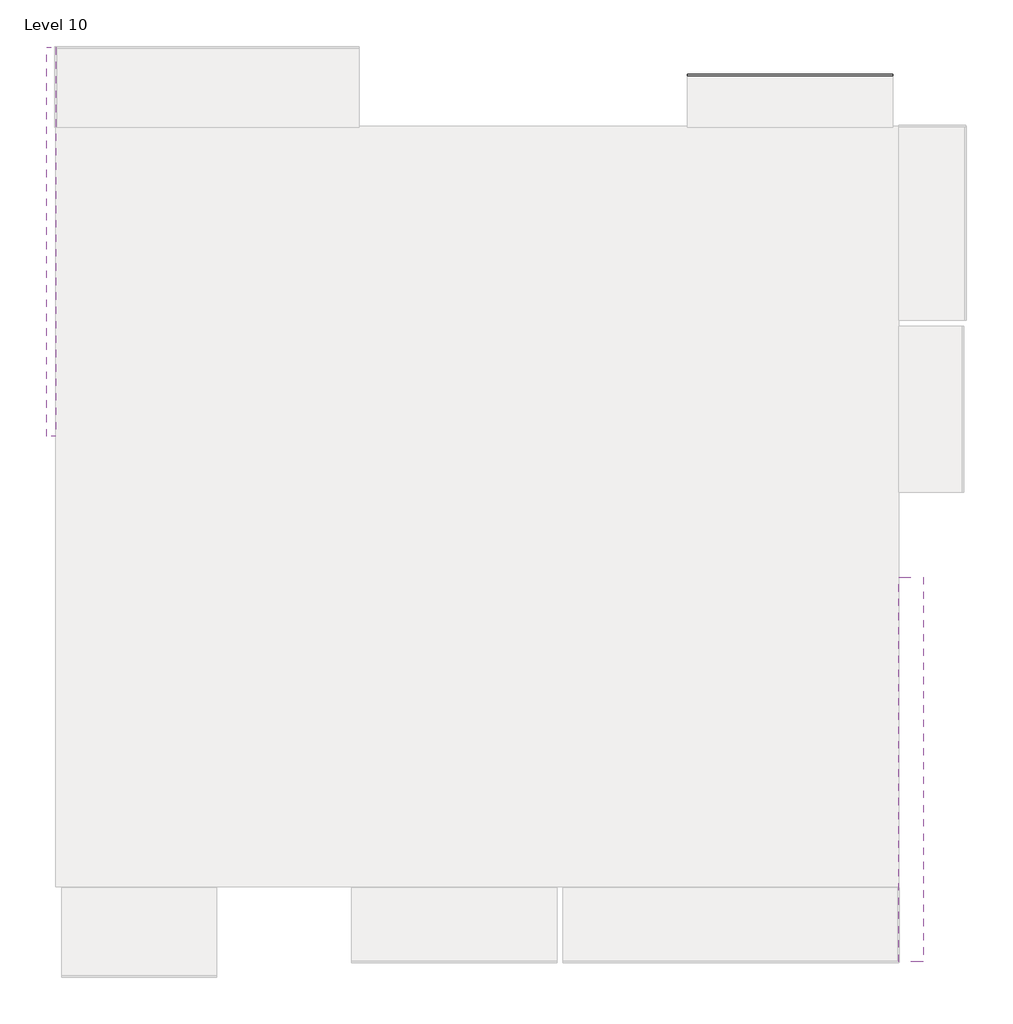
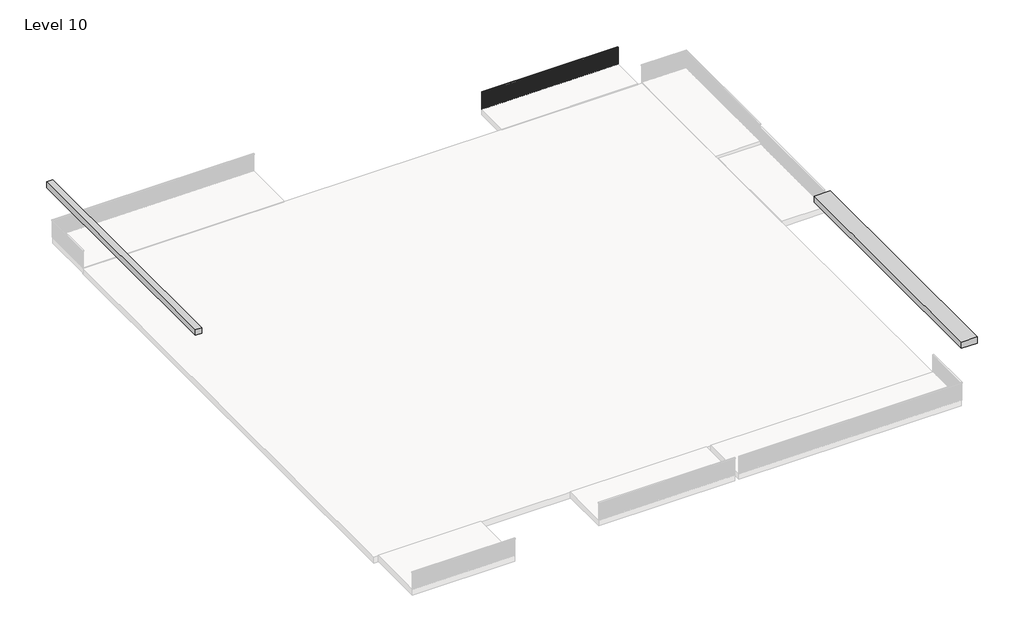
# One storey, part 5 of 5: 2 proxies, 1 railing.
"""IFC4 building model written with IfcOpenShell, lengths in millimetres."""

from ifc_helpers import new_model, si_unit, frame, origin, place, context, project, spatial, polyline, outline, extrude, transform, mapped, element, save
from components import generic_models_7_generic_models_4_98acaeb1, generic_models_10_generic_models_8_4a409525

model = new_model("IFC4")

# Units and contexts
model_context = context("Model", 3, world=origin())
ifc_project = project(units=[si_unit("LENGTHUNIT", "METRE", prefix="MILLI")], contexts=[model_context])

# Site, building, storey
site = spatial("IfcSite", under=ifc_project)
building = spatial("IfcBuilding", under=site)
storey = spatial("IfcBuildingStorey", under=building, Name="Level 10", Elevation=12496.8)

# Proxies
placement = place(None, origin())
generic_models_7_generic_models_4_shape = generic_models_7_generic_models_4_98acaeb1(model_context)
element("IfcBuildingElementProxy", 1, Name="Generic Models 7 : Generic Models 4", ObjectType="Generic Models 7 : Generic Models 4", at=placement, inside=storey, context=model_context, shape_type="MappedRepresentation", body=[
    mapped(generic_models_7_generic_models_4_shape, transform((0.0, -159.6595923, 9459.6818533), x_axis=(1.0, 0.0, 0.0), y_axis=(0.0, 1.0, 0.0), z_axis=(0.0, 0.0, 1.0))),
])
generic_models_10_generic_models_8_shape = generic_models_10_generic_models_8_4a409525(model_context)
element("IfcBuildingElementProxy", 2, Name="Generic Models 9 : Generic Models 8", ObjectType="Generic Models 9 : Generic Models 8", at=placement, inside=storey, context=model_context, shape_type="MappedRepresentation", body=[
    mapped(generic_models_10_generic_models_8_shape, transform((0.0, 0.0, -3200.4), x_axis=(1.0, 0.0, 0.0), y_axis=(0.0, 1.0, 0.0), z_axis=(0.0, 0.0, 1.0))),
])

# Railing
element("IfcRailing", 3, ObjectType="Handrail - Rectangular", at=placement, inside=storey, context=model_context, shape_type="SweptSolid", body=[
    extrude(outline(polyline([(7096.1361222, 16470.4237525), (7096.1361222, 16521.2237525), (13903.3361222, 16521.2237525), (13903.3361222, 16470.4237525), (7096.1361222, 16470.4237525)])), frame((0.0, 0.0, 13360.4), z_axis=(0.0, 0.0, 1.0), x_axis=(1.0, 0.0, 0.0)), (0.0, 0.0, 1.0), 50.8),
    extrude(outline(polyline([(13792.2111222, 16486.2987525), (13792.2111222, 16505.3487525), (13811.2611222, 16505.3487525), (13811.2611222, 16486.2987525), (13792.2111222, 16486.2987525)])), frame((0.0, 0.0, 12496.8), z_axis=(0.0, 0.0, 1.0), x_axis=(1.0, 0.0, 0.0)), (0.0, 0.0, 1.0), 863.6),
    extrude(outline(polyline([(13690.6111222, 16486.2987525), (13690.6111222, 16505.3487525), (13709.6611222, 16505.3487525), (13709.6611222, 16486.2987525), (13690.6111222, 16486.2987525)])), frame((0.0, 0.0, 12496.8), z_axis=(0.0, 0.0, 1.0), x_axis=(1.0, 0.0, 0.0)), (0.0, 0.0, 1.0), 863.6),
    extrude(outline(polyline([(13589.0111222, 16486.2987525), (13589.0111222, 16505.3487525), (13608.0611222, 16505.3487525), (13608.0611222, 16486.2987525), (13589.0111222, 16486.2987525)])), frame((0.0, 0.0, 12496.8), z_axis=(0.0, 0.0, 1.0), x_axis=(1.0, 0.0, 0.0)), (0.0, 0.0, 1.0), 863.6),
    extrude(outline(polyline([(13487.4111222, 16486.2987525), (13487.4111222, 16505.3487525), (13506.4611222, 16505.3487525), (13506.4611222, 16486.2987525), (13487.4111222, 16486.2987525)])), frame((0.0, 0.0, 12496.8), z_axis=(0.0, 0.0, 1.0), x_axis=(1.0, 0.0, 0.0)), (0.0, 0.0, 1.0), 863.6),
    extrude(outline(polyline([(13385.8111222, 16486.2987525), (13385.8111222, 16505.3487525), (13404.8611222, 16505.3487525), (13404.8611222, 16486.2987525), (13385.8111222, 16486.2987525)])), frame((0.0, 0.0, 12496.8), z_axis=(0.0, 0.0, 1.0), x_axis=(1.0, 0.0, 0.0)), (0.0, 0.0, 1.0), 863.6),
    extrude(outline(polyline([(13284.2111222, 16486.2987525), (13284.2111222, 16505.3487525), (13303.2611222, 16505.3487525), (13303.2611222, 16486.2987525), (13284.2111222, 16486.2987525)])), frame((0.0, 0.0, 12496.8), z_axis=(0.0, 0.0, 1.0), x_axis=(1.0, 0.0, 0.0)), (0.0, 0.0, 1.0), 863.6),
    extrude(outline(polyline([(13182.6111222, 16486.2987525), (13182.6111222, 16505.3487525), (13201.6611222, 16505.3487525), (13201.6611222, 16486.2987525), (13182.6111222, 16486.2987525)])), frame((0.0, 0.0, 12496.8), z_axis=(0.0, 0.0, 1.0), x_axis=(1.0, 0.0, 0.0)), (0.0, 0.0, 1.0), 863.6),
    extrude(outline(polyline([(13081.0111222, 16486.2987525), (13081.0111222, 16505.3487525), (13100.0611222, 16505.3487525), (13100.0611222, 16486.2987525), (13081.0111222, 16486.2987525)])), frame((0.0, 0.0, 12496.8), z_axis=(0.0, 0.0, 1.0), x_axis=(1.0, 0.0, 0.0)), (0.0, 0.0, 1.0), 863.6),
    extrude(outline(polyline([(12979.4111222, 16486.2987525), (12979.4111222, 16505.3487525), (12998.4611222, 16505.3487525), (12998.4611222, 16486.2987525), (12979.4111222, 16486.2987525)])), frame((0.0, 0.0, 12496.8), z_axis=(0.0, 0.0, 1.0), x_axis=(1.0, 0.0, 0.0)), (0.0, 0.0, 1.0), 863.6),
    extrude(outline(polyline([(12877.8111222, 16486.2987525), (12877.8111222, 16505.3487525), (12896.8611222, 16505.3487525), (12896.8611222, 16486.2987525), (12877.8111222, 16486.2987525)])), frame((0.0, 0.0, 12496.8), z_axis=(0.0, 0.0, 1.0), x_axis=(1.0, 0.0, 0.0)), (0.0, 0.0, 1.0), 863.6),
    extrude(outline(polyline([(12776.2111222, 16486.2987525), (12776.2111222, 16505.3487525), (12795.2611222, 16505.3487525), (12795.2611222, 16486.2987525), (12776.2111222, 16486.2987525)])), frame((0.0, 0.0, 12496.8), z_axis=(0.0, 0.0, 1.0), x_axis=(1.0, 0.0, 0.0)), (0.0, 0.0, 1.0), 863.6),
    extrude(outline(polyline([(12674.6111222, 16486.2987525), (12674.6111222, 16505.3487525), (12693.6611222, 16505.3487525), (12693.6611222, 16486.2987525), (12674.6111222, 16486.2987525)])), frame((0.0, 0.0, 12496.8), z_axis=(0.0, 0.0, 1.0), x_axis=(1.0, 0.0, 0.0)), (0.0, 0.0, 1.0), 863.6),
    extrude(outline(polyline([(12573.0111222, 16486.2987525), (12573.0111222, 16505.3487525), (12592.0611222, 16505.3487525), (12592.0611222, 16486.2987525), (12573.0111222, 16486.2987525)])), frame((0.0, 0.0, 12496.8), z_axis=(0.0, 0.0, 1.0), x_axis=(1.0, 0.0, 0.0)), (0.0, 0.0, 1.0), 863.6),
    extrude(outline(polyline([(12471.4111222, 16486.2987525), (12471.4111222, 16505.3487525), (12490.4611222, 16505.3487525), (12490.4611222, 16486.2987525), (12471.4111222, 16486.2987525)])), frame((0.0, 0.0, 12496.8), z_axis=(0.0, 0.0, 1.0), x_axis=(1.0, 0.0, 0.0)), (0.0, 0.0, 1.0), 863.6),
    extrude(outline(polyline([(12369.8111222, 16486.2987525), (12369.8111222, 16505.3487525), (12388.8611222, 16505.3487525), (12388.8611222, 16486.2987525), (12369.8111222, 16486.2987525)])), frame((0.0, 0.0, 12496.8), z_axis=(0.0, 0.0, 1.0), x_axis=(1.0, 0.0, 0.0)), (0.0, 0.0, 1.0), 863.6),
    extrude(outline(polyline([(12268.2111222, 16486.2987525), (12268.2111222, 16505.3487525), (12287.2611222, 16505.3487525), (12287.2611222, 16486.2987525), (12268.2111222, 16486.2987525)])), frame((0.0, 0.0, 12496.8), z_axis=(0.0, 0.0, 1.0), x_axis=(1.0, 0.0, 0.0)), (0.0, 0.0, 1.0), 863.6),
    extrude(outline(polyline([(12166.6111222, 16486.2987525), (12166.6111222, 16505.3487525), (12185.6611222, 16505.3487525), (12185.6611222, 16486.2987525), (12166.6111222, 16486.2987525)])), frame((0.0, 0.0, 12496.8), z_axis=(0.0, 0.0, 1.0), x_axis=(1.0, 0.0, 0.0)), (0.0, 0.0, 1.0), 863.6),
    extrude(outline(polyline([(12065.0111222, 16486.2987525), (12065.0111222, 16505.3487525), (12084.0611222, 16505.3487525), (12084.0611222, 16486.2987525), (12065.0111222, 16486.2987525)])), frame((0.0, 0.0, 12496.8), z_axis=(0.0, 0.0, 1.0), x_axis=(1.0, 0.0, 0.0)), (0.0, 0.0, 1.0), 863.6),
    extrude(outline(polyline([(11963.4111222, 16486.2987525), (11963.4111222, 16505.3487525), (11982.4611222, 16505.3487525), (11982.4611222, 16486.2987525), (11963.4111222, 16486.2987525)])), frame((0.0, 0.0, 12496.8), z_axis=(0.0, 0.0, 1.0), x_axis=(1.0, 0.0, 0.0)), (0.0, 0.0, 1.0), 863.6),
    extrude(outline(polyline([(11861.8111222, 16486.2987525), (11861.8111222, 16505.3487525), (11880.8611222, 16505.3487525), (11880.8611222, 16486.2987525), (11861.8111222, 16486.2987525)])), frame((0.0, 0.0, 12496.8), z_axis=(0.0, 0.0, 1.0), x_axis=(1.0, 0.0, 0.0)), (0.0, 0.0, 1.0), 863.6),
    extrude(outline(polyline([(11760.2111222, 16486.2987525), (11760.2111222, 16505.3487525), (11779.2611222, 16505.3487525), (11779.2611222, 16486.2987525), (11760.2111222, 16486.2987525)])), frame((0.0, 0.0, 12496.8), z_axis=(0.0, 0.0, 1.0), x_axis=(1.0, 0.0, 0.0)), (0.0, 0.0, 1.0), 863.6),
    extrude(outline(polyline([(11658.6111222, 16486.2987525), (11658.6111222, 16505.3487525), (11677.6611222, 16505.3487525), (11677.6611222, 16486.2987525), (11658.6111222, 16486.2987525)])), frame((0.0, 0.0, 12496.8), z_axis=(0.0, 0.0, 1.0), x_axis=(1.0, 0.0, 0.0)), (0.0, 0.0, 1.0), 863.6),
    extrude(outline(polyline([(11557.0111222, 16486.2987525), (11557.0111222, 16505.3487525), (11576.0611222, 16505.3487525), (11576.0611222, 16486.2987525), (11557.0111222, 16486.2987525)])), frame((0.0, 0.0, 12496.8), z_axis=(0.0, 0.0, 1.0), x_axis=(1.0, 0.0, 0.0)), (0.0, 0.0, 1.0), 863.6),
    extrude(outline(polyline([(11455.4111222, 16486.2987525), (11455.4111222, 16505.3487525), (11474.4611222, 16505.3487525), (11474.4611222, 16486.2987525), (11455.4111222, 16486.2987525)])), frame((0.0, 0.0, 12496.8), z_axis=(0.0, 0.0, 1.0), x_axis=(1.0, 0.0, 0.0)), (0.0, 0.0, 1.0), 863.6),
    extrude(outline(polyline([(11353.8111222, 16486.2987525), (11353.8111222, 16505.3487525), (11372.8611222, 16505.3487525), (11372.8611222, 16486.2987525), (11353.8111222, 16486.2987525)])), frame((0.0, 0.0, 12496.8), z_axis=(0.0, 0.0, 1.0), x_axis=(1.0, 0.0, 0.0)), (0.0, 0.0, 1.0), 863.6),
    extrude(outline(polyline([(11252.2111222, 16486.2987525), (11252.2111222, 16505.3487525), (11271.2611222, 16505.3487525), (11271.2611222, 16486.2987525), (11252.2111222, 16486.2987525)])), frame((0.0, 0.0, 12496.8), z_axis=(0.0, 0.0, 1.0), x_axis=(1.0, 0.0, 0.0)), (0.0, 0.0, 1.0), 863.6),
    extrude(outline(polyline([(11150.6111222, 16486.2987525), (11150.6111222, 16505.3487525), (11169.6611222, 16505.3487525), (11169.6611222, 16486.2987525), (11150.6111222, 16486.2987525)])), frame((0.0, 0.0, 12496.8), z_axis=(0.0, 0.0, 1.0), x_axis=(1.0, 0.0, 0.0)), (0.0, 0.0, 1.0), 863.6),
    extrude(outline(polyline([(11049.0111222, 16486.2987525), (11049.0111222, 16505.3487525), (11068.0611222, 16505.3487525), (11068.0611222, 16486.2987525), (11049.0111222, 16486.2987525)])), frame((0.0, 0.0, 12496.8), z_axis=(0.0, 0.0, 1.0), x_axis=(1.0, 0.0, 0.0)), (0.0, 0.0, 1.0), 863.6),
    extrude(outline(polyline([(10947.4111222, 16486.2987525), (10947.4111222, 16505.3487525), (10966.4611222, 16505.3487525), (10966.4611222, 16486.2987525), (10947.4111222, 16486.2987525)])), frame((0.0, 0.0, 12496.8), z_axis=(0.0, 0.0, 1.0), x_axis=(1.0, 0.0, 0.0)), (0.0, 0.0, 1.0), 863.6),
    extrude(outline(polyline([(10845.8111222, 16486.2987525), (10845.8111222, 16505.3487525), (10864.8611222, 16505.3487525), (10864.8611222, 16486.2987525), (10845.8111222, 16486.2987525)])), frame((0.0, 0.0, 12496.8), z_axis=(0.0, 0.0, 1.0), x_axis=(1.0, 0.0, 0.0)), (0.0, 0.0, 1.0), 863.6),
    extrude(outline(polyline([(10744.2111222, 16486.2987525), (10744.2111222, 16505.3487525), (10763.2611222, 16505.3487525), (10763.2611222, 16486.2987525), (10744.2111222, 16486.2987525)])), frame((0.0, 0.0, 12496.8), z_axis=(0.0, 0.0, 1.0), x_axis=(1.0, 0.0, 0.0)), (0.0, 0.0, 1.0), 863.6),
    extrude(outline(polyline([(10642.6111222, 16486.2987525), (10642.6111222, 16505.3487525), (10661.6611222, 16505.3487525), (10661.6611222, 16486.2987525), (10642.6111222, 16486.2987525)])), frame((0.0, 0.0, 12496.8), z_axis=(0.0, 0.0, 1.0), x_axis=(1.0, 0.0, 0.0)), (0.0, 0.0, 1.0), 863.6),
    extrude(outline(polyline([(10541.0111222, 16486.2987525), (10541.0111222, 16505.3487525), (10560.0611222, 16505.3487525), (10560.0611222, 16486.2987525), (10541.0111222, 16486.2987525)])), frame((0.0, 0.0, 12496.8), z_axis=(0.0, 0.0, 1.0), x_axis=(1.0, 0.0, 0.0)), (0.0, 0.0, 1.0), 863.6),
    extrude(outline(polyline([(10439.4111222, 16486.2987525), (10439.4111222, 16505.3487525), (10458.4611222, 16505.3487525), (10458.4611222, 16486.2987525), (10439.4111222, 16486.2987525)])), frame((0.0, 0.0, 12496.8), z_axis=(0.0, 0.0, 1.0), x_axis=(1.0, 0.0, 0.0)), (0.0, 0.0, 1.0), 863.6),
    extrude(outline(polyline([(10337.8111222, 16486.2987525), (10337.8111222, 16505.3487525), (10356.8611222, 16505.3487525), (10356.8611222, 16486.2987525), (10337.8111222, 16486.2987525)])), frame((0.0, 0.0, 12496.8), z_axis=(0.0, 0.0, 1.0), x_axis=(1.0, 0.0, 0.0)), (0.0, 0.0, 1.0), 863.6),
    extrude(outline(polyline([(10236.2111222, 16486.2987525), (10236.2111222, 16505.3487525), (10255.2611222, 16505.3487525), (10255.2611222, 16486.2987525), (10236.2111222, 16486.2987525)])), frame((0.0, 0.0, 12496.8), z_axis=(0.0, 0.0, 1.0), x_axis=(1.0, 0.0, 0.0)), (0.0, 0.0, 1.0), 863.6),
    extrude(outline(polyline([(10134.6111222, 16486.2987525), (10134.6111222, 16505.3487525), (10153.6611222, 16505.3487525), (10153.6611222, 16486.2987525), (10134.6111222, 16486.2987525)])), frame((0.0, 0.0, 12496.8), z_axis=(0.0, 0.0, 1.0), x_axis=(1.0, 0.0, 0.0)), (0.0, 0.0, 1.0), 863.6),
    extrude(outline(polyline([(10033.0111222, 16486.2987525), (10033.0111222, 16505.3487525), (10052.0611222, 16505.3487525), (10052.0611222, 16486.2987525), (10033.0111222, 16486.2987525)])), frame((0.0, 0.0, 12496.8), z_axis=(0.0, 0.0, 1.0), x_axis=(1.0, 0.0, 0.0)), (0.0, 0.0, 1.0), 863.6),
    extrude(outline(polyline([(9931.4111222, 16486.2987525), (9931.4111222, 16505.3487525), (9950.4611222, 16505.3487525), (9950.4611222, 16486.2987525), (9931.4111222, 16486.2987525)])), frame((0.0, 0.0, 12496.8), z_axis=(0.0, 0.0, 1.0), x_axis=(1.0, 0.0, 0.0)), (0.0, 0.0, 1.0), 863.6),
    extrude(outline(polyline([(9829.8111222, 16486.2987525), (9829.8111222, 16505.3487525), (9848.8611222, 16505.3487525), (9848.8611222, 16486.2987525), (9829.8111222, 16486.2987525)])), frame((0.0, 0.0, 12496.8), z_axis=(0.0, 0.0, 1.0), x_axis=(1.0, 0.0, 0.0)), (0.0, 0.0, 1.0), 863.6),
    extrude(outline(polyline([(9728.2111222, 16486.2987525), (9728.2111222, 16505.3487525), (9747.2611222, 16505.3487525), (9747.2611222, 16486.2987525), (9728.2111222, 16486.2987525)])), frame((0.0, 0.0, 12496.8), z_axis=(0.0, 0.0, 1.0), x_axis=(1.0, 0.0, 0.0)), (0.0, 0.0, 1.0), 863.6),
    extrude(outline(polyline([(9626.6111222, 16486.2987525), (9626.6111222, 16505.3487525), (9645.6611222, 16505.3487525), (9645.6611222, 16486.2987525), (9626.6111222, 16486.2987525)])), frame((0.0, 0.0, 12496.8), z_axis=(0.0, 0.0, 1.0), x_axis=(1.0, 0.0, 0.0)), (0.0, 0.0, 1.0), 863.6),
    extrude(outline(polyline([(9525.0111222, 16486.2987525), (9525.0111222, 16505.3487525), (9544.0611222, 16505.3487525), (9544.0611222, 16486.2987525), (9525.0111222, 16486.2987525)])), frame((0.0, 0.0, 12496.8), z_axis=(0.0, 0.0, 1.0), x_axis=(1.0, 0.0, 0.0)), (0.0, 0.0, 1.0), 863.6),
    extrude(outline(polyline([(9423.4111222, 16486.2987525), (9423.4111222, 16505.3487525), (9442.4611222, 16505.3487525), (9442.4611222, 16486.2987525), (9423.4111222, 16486.2987525)])), frame((0.0, 0.0, 12496.8), z_axis=(0.0, 0.0, 1.0), x_axis=(1.0, 0.0, 0.0)), (0.0, 0.0, 1.0), 863.6),
    extrude(outline(polyline([(9321.8111222, 16486.2987525), (9321.8111222, 16505.3487525), (9340.8611222, 16505.3487525), (9340.8611222, 16486.2987525), (9321.8111222, 16486.2987525)])), frame((0.0, 0.0, 12496.8), z_axis=(0.0, 0.0, 1.0), x_axis=(1.0, 0.0, 0.0)), (0.0, 0.0, 1.0), 863.6),
    extrude(outline(polyline([(9220.2111222, 16486.2987525), (9220.2111222, 16505.3487525), (9239.2611222, 16505.3487525), (9239.2611222, 16486.2987525), (9220.2111222, 16486.2987525)])), frame((0.0, 0.0, 12496.8), z_axis=(0.0, 0.0, 1.0), x_axis=(1.0, 0.0, 0.0)), (0.0, 0.0, 1.0), 863.6),
    extrude(outline(polyline([(9118.6111222, 16486.2987525), (9118.6111222, 16505.3487525), (9137.6611222, 16505.3487525), (9137.6611222, 16486.2987525), (9118.6111222, 16486.2987525)])), frame((0.0, 0.0, 12496.8), z_axis=(0.0, 0.0, 1.0), x_axis=(1.0, 0.0, 0.0)), (0.0, 0.0, 1.0), 863.6),
    extrude(outline(polyline([(9017.0111222, 16486.2987525), (9017.0111222, 16505.3487525), (9036.0611222, 16505.3487525), (9036.0611222, 16486.2987525), (9017.0111222, 16486.2987525)])), frame((0.0, 0.0, 12496.8), z_axis=(0.0, 0.0, 1.0), x_axis=(1.0, 0.0, 0.0)), (0.0, 0.0, 1.0), 863.6),
    extrude(outline(polyline([(8915.4111222, 16486.2987525), (8915.4111222, 16505.3487525), (8934.4611222, 16505.3487525), (8934.4611222, 16486.2987525), (8915.4111222, 16486.2987525)])), frame((0.0, 0.0, 12496.8), z_axis=(0.0, 0.0, 1.0), x_axis=(1.0, 0.0, 0.0)), (0.0, 0.0, 1.0), 863.6),
    extrude(outline(polyline([(8813.8111222, 16486.2987525), (8813.8111222, 16505.3487525), (8832.8611222, 16505.3487525), (8832.8611222, 16486.2987525), (8813.8111222, 16486.2987525)])), frame((0.0, 0.0, 12496.8), z_axis=(0.0, 0.0, 1.0), x_axis=(1.0, 0.0, 0.0)), (0.0, 0.0, 1.0), 863.6),
    extrude(outline(polyline([(8712.2111222, 16486.2987525), (8712.2111222, 16505.3487525), (8731.2611222, 16505.3487525), (8731.2611222, 16486.2987525), (8712.2111222, 16486.2987525)])), frame((0.0, 0.0, 12496.8), z_axis=(0.0, 0.0, 1.0), x_axis=(1.0, 0.0, 0.0)), (0.0, 0.0, 1.0), 863.6),
    extrude(outline(polyline([(8610.6111222, 16486.2987525), (8610.6111222, 16505.3487525), (8629.6611222, 16505.3487525), (8629.6611222, 16486.2987525), (8610.6111222, 16486.2987525)])), frame((0.0, 0.0, 12496.8), z_axis=(0.0, 0.0, 1.0), x_axis=(1.0, 0.0, 0.0)), (0.0, 0.0, 1.0), 863.6),
    extrude(outline(polyline([(8509.0111222, 16486.2987525), (8509.0111222, 16505.3487525), (8528.0611222, 16505.3487525), (8528.0611222, 16486.2987525), (8509.0111222, 16486.2987525)])), frame((0.0, 0.0, 12496.8), z_axis=(0.0, 0.0, 1.0), x_axis=(1.0, 0.0, 0.0)), (0.0, 0.0, 1.0), 863.6),
    extrude(outline(polyline([(8407.4111222, 16486.2987525), (8407.4111222, 16505.3487525), (8426.4611222, 16505.3487525), (8426.4611222, 16486.2987525), (8407.4111222, 16486.2987525)])), frame((0.0, 0.0, 12496.8), z_axis=(0.0, 0.0, 1.0), x_axis=(1.0, 0.0, 0.0)), (0.0, 0.0, 1.0), 863.6),
    extrude(outline(polyline([(8305.8111222, 16486.2987525), (8305.8111222, 16505.3487525), (8324.8611222, 16505.3487525), (8324.8611222, 16486.2987525), (8305.8111222, 16486.2987525)])), frame((0.0, 0.0, 12496.8), z_axis=(0.0, 0.0, 1.0), x_axis=(1.0, 0.0, 0.0)), (0.0, 0.0, 1.0), 863.6),
    extrude(outline(polyline([(8204.2111222, 16486.2987525), (8204.2111222, 16505.3487525), (8223.2611222, 16505.3487525), (8223.2611222, 16486.2987525), (8204.2111222, 16486.2987525)])), frame((0.0, 0.0, 12496.8), z_axis=(0.0, 0.0, 1.0), x_axis=(1.0, 0.0, 0.0)), (0.0, 0.0, 1.0), 863.6),
    extrude(outline(polyline([(8102.6111222, 16486.2987525), (8102.6111222, 16505.3487525), (8121.6611222, 16505.3487525), (8121.6611222, 16486.2987525), (8102.6111222, 16486.2987525)])), frame((0.0, 0.0, 12496.8), z_axis=(0.0, 0.0, 1.0), x_axis=(1.0, 0.0, 0.0)), (0.0, 0.0, 1.0), 863.6),
    extrude(outline(polyline([(8001.0111222, 16486.2987525), (8001.0111222, 16505.3487525), (8020.0611222, 16505.3487525), (8020.0611222, 16486.2987525), (8001.0111222, 16486.2987525)])), frame((0.0, 0.0, 12496.8), z_axis=(0.0, 0.0, 1.0), x_axis=(1.0, 0.0, 0.0)), (0.0, 0.0, 1.0), 863.6),
    extrude(outline(polyline([(7899.4111222, 16486.2987525), (7899.4111222, 16505.3487525), (7918.4611222, 16505.3487525), (7918.4611222, 16486.2987525), (7899.4111222, 16486.2987525)])), frame((0.0, 0.0, 12496.8), z_axis=(0.0, 0.0, 1.0), x_axis=(1.0, 0.0, 0.0)), (0.0, 0.0, 1.0), 863.6),
    extrude(outline(polyline([(7797.8111222, 16486.2987525), (7797.8111222, 16505.3487525), (7816.8611222, 16505.3487525), (7816.8611222, 16486.2987525), (7797.8111222, 16486.2987525)])), frame((0.0, 0.0, 12496.8), z_axis=(0.0, 0.0, 1.0), x_axis=(1.0, 0.0, 0.0)), (0.0, 0.0, 1.0), 863.6),
    extrude(outline(polyline([(7696.2111222, 16486.2987525), (7696.2111222, 16505.3487525), (7715.2611222, 16505.3487525), (7715.2611222, 16486.2987525), (7696.2111222, 16486.2987525)])), frame((0.0, 0.0, 12496.8), z_axis=(0.0, 0.0, 1.0), x_axis=(1.0, 0.0, 0.0)), (0.0, 0.0, 1.0), 863.6),
    extrude(outline(polyline([(7594.6111222, 16486.2987525), (7594.6111222, 16505.3487525), (7613.6611222, 16505.3487525), (7613.6611222, 16486.2987525), (7594.6111222, 16486.2987525)])), frame((0.0, 0.0, 12496.8), z_axis=(0.0, 0.0, 1.0), x_axis=(1.0, 0.0, 0.0)), (0.0, 0.0, 1.0), 863.6),
    extrude(outline(polyline([(7493.0111222, 16486.2987525), (7493.0111222, 16505.3487525), (7512.0611222, 16505.3487525), (7512.0611222, 16486.2987525), (7493.0111222, 16486.2987525)])), frame((0.0, 0.0, 12496.8), z_axis=(0.0, 0.0, 1.0), x_axis=(1.0, 0.0, 0.0)), (0.0, 0.0, 1.0), 863.6),
    extrude(outline(polyline([(7391.4111222, 16486.2987525), (7391.4111222, 16505.3487525), (7410.4611222, 16505.3487525), (7410.4611222, 16486.2987525), (7391.4111222, 16486.2987525)])), frame((0.0, 0.0, 12496.8), z_axis=(0.0, 0.0, 1.0), x_axis=(1.0, 0.0, 0.0)), (0.0, 0.0, 1.0), 863.6),
    extrude(outline(polyline([(7289.8111222, 16486.2987525), (7289.8111222, 16505.3487525), (7308.8611222, 16505.3487525), (7308.8611222, 16486.2987525), (7289.8111222, 16486.2987525)])), frame((0.0, 0.0, 12496.8), z_axis=(0.0, 0.0, 1.0), x_axis=(1.0, 0.0, 0.0)), (0.0, 0.0, 1.0), 863.6),
    extrude(outline(polyline([(7188.2111222, 16486.2987525), (7188.2111222, 16505.3487525), (7207.2611222, 16505.3487525), (7207.2611222, 16486.2987525), (7188.2111222, 16486.2987525)])), frame((0.0, 0.0, 12496.8), z_axis=(0.0, 0.0, 1.0), x_axis=(1.0, 0.0, 0.0)), (0.0, 0.0, 1.0), 863.6),
    extrude(outline(polyline([(13884.2861222, 16486.2987525), (13884.2861222, 16505.3487525), (13903.3361222, 16505.3487525), (13903.3361222, 16486.2987525), (13884.2861222, 16486.2987525)])), frame((0.0, 0.0, 12496.8), z_axis=(0.0, 0.0, 1.0), x_axis=(1.0, 0.0, 0.0)), (0.0, 0.0, 1.0), 863.6),
    extrude(outline(polyline([(7096.1361222, 16486.2987525), (7096.1361222, 16505.3487525), (7115.1861222, 16505.3487525), (7115.1861222, 16486.2987525), (7096.1361222, 16486.2987525)])), frame((0.0, 0.0, 12496.8), z_axis=(0.0, 0.0, 1.0), x_axis=(1.0, 0.0, 0.0)), (0.0, 0.0, 1.0), 863.6),
])

save(model, "model.ifc")

# Revit data of these elements
# Type "Handrail - Rectangular"
#   Assembly Code = "C2010400"
#   built-in parameter 1008612 = 0.0416667 (stored number, unit not read)
#   built-in parameter 1008611 = 0.0416667 (stored number, unit not read)
#   built-in parameter 1008609 = 0.333333 (stored number, unit not read)
#   built-in parameter 1008604 = 0.166667 (stored number, unit not read)
#   built-in parameter 1008603 = 0.166667 (stored number, unit not read)
#   Railing Height = 3' - 0"
#   built-in parameter 1008630 = 2
#   built-in parameter 1008610 = 2
#   built-in parameter 1008618 = Baluster - Square : 3/4"
# Element 1 (IfcBuildingElementProxy, "Generic Models 7 : Generic Models 4")
#   Phase Created = New Construction
# Element 2 (IfcBuildingElementProxy, "Generic Models 9 : Generic Models 8")
#   Phase Created = New Construction
# Element 3 (IfcRailing, "Handrail - Rectangular")
#   Phase Created = New Construction
